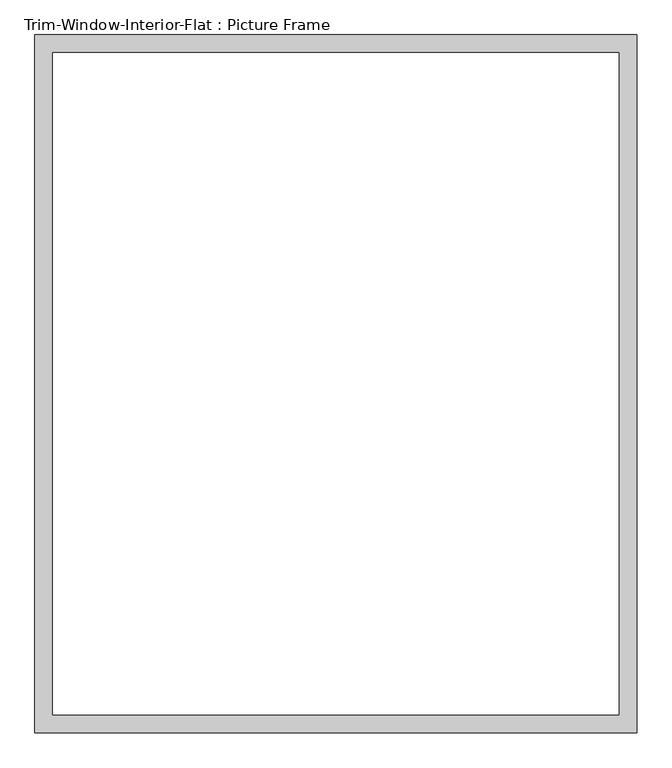
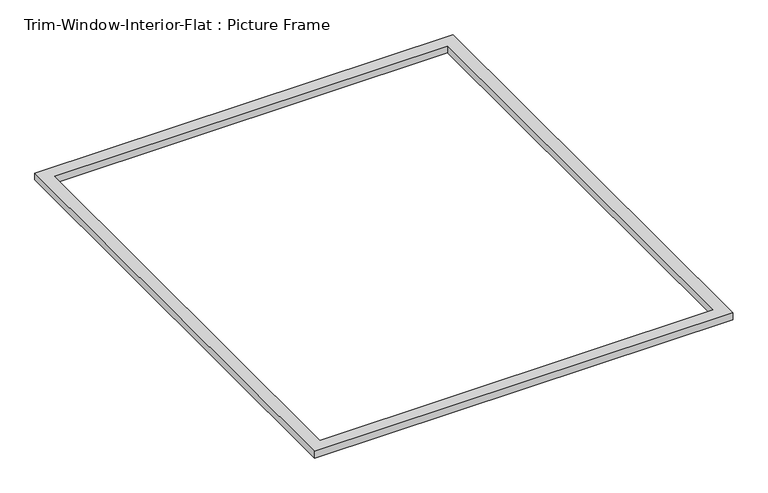
"""IFC4 building model written with IfcOpenShell, lengths in millimetres: proxy geometry, Trim-Window-Interior-Flat : Picture Frame."""

from ifc_helpers import new_model, si_unit, origin, origin_with_axes, place, context, project, spatial, polyline, outline, extrude, source, transform, mapped, element, save


def trim_window_interior_flat_picture_frame_e62f86b4(model_context):
    return source(origin(), model_context, "Body", "SweptSolid", [
        extrude(outline(polyline([(958.85, 44.45), (958.85, -2178.05), (-958.85, -2178.05), (-958.85, 44.45), (958.85, 44.45)]), holes=[polyline([(901.7, -12.7), (-901.7, -12.7), (-901.7, -2120.9), (901.7, -2120.9), (901.7, -12.7)])]), origin_with_axes(), (0.0, 0.0, 1.0), 31.75),
    ])


if __name__ == "__main__":
    model = new_model("IFC4")
    model_context = context("Model", 3, world=origin())
    ifc_project = project(units=[si_unit("LENGTHUNIT", "METRE", prefix="MILLI")], contexts=[model_context])
    site = spatial("IfcSite", under=ifc_project)
    building = spatial("IfcBuilding", under=site)
    placement = place(None, origin())
    trim_window_interior_flat_picture_frame_shape = trim_window_interior_flat_picture_frame_e62f86b4(model_context)
    element("IfcBuildingElementProxy", 1, Name="Trim-Window-Interior-Flat : Picture Frame", ObjectType="Trim-Window-Interior-Flat : Picture Frame", at=placement, inside=building, context=model_context, shape_type="MappedRepresentation", body=[
        mapped(trim_window_interior_flat_picture_frame_shape, transform((0.0, 0.0, 0.0), x_axis=(1.0, 0.0, 0.0), y_axis=(0.0, 1.0, 0.0), z_axis=(0.0, 0.0, 1.0))),
    ])
    save(model, "model.ifc")

# Revit data of these elements
# Type "Trim-Window-Interior-Flat : Picture Frame"
#   Trim Thickness_Picture Frame = 0' - 1 1/4"
#   Trim Width = 0' - 2 1/4"
#   Trim Thickness_with Sill = 0' - 0 3/4"
#   Sill Thickness = 0' - 1 1/4"
#   Opening Width [instance default] = 2' - 0"
#   Opening Height [instance default] = 3' - 0"
#   Default Elevation = 4' - 0"
#   Sill = no
#   Picture Frame = yes
#   Trim Material [instance default] = none
# Element 1 (IfcBuildingElementProxy, "Trim-Window-Interior-Flat : Picture Frame")
#   Opening Width = 6' - 0"
#   Opening Height = 7' - 0"
#   Trim Material = Wood - Stained
#   Materials on its faces: "Wood - Stained"
# Materials
#   "Wood - Stained": class "Wood", colour RGB 224 178 126, transparency 0, Cost = 0
